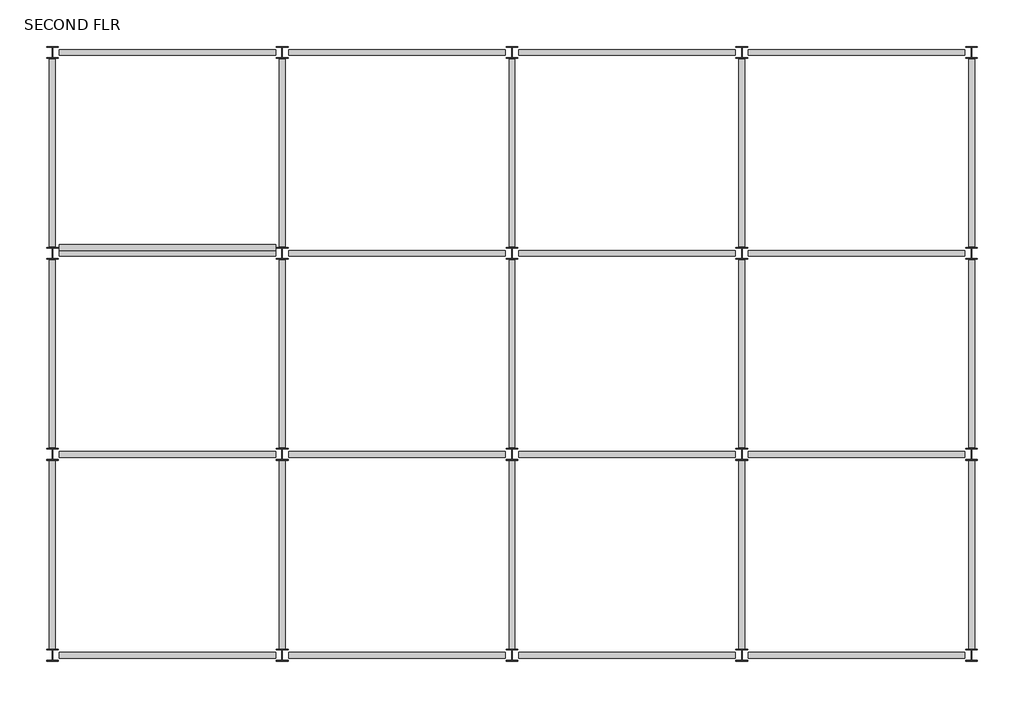
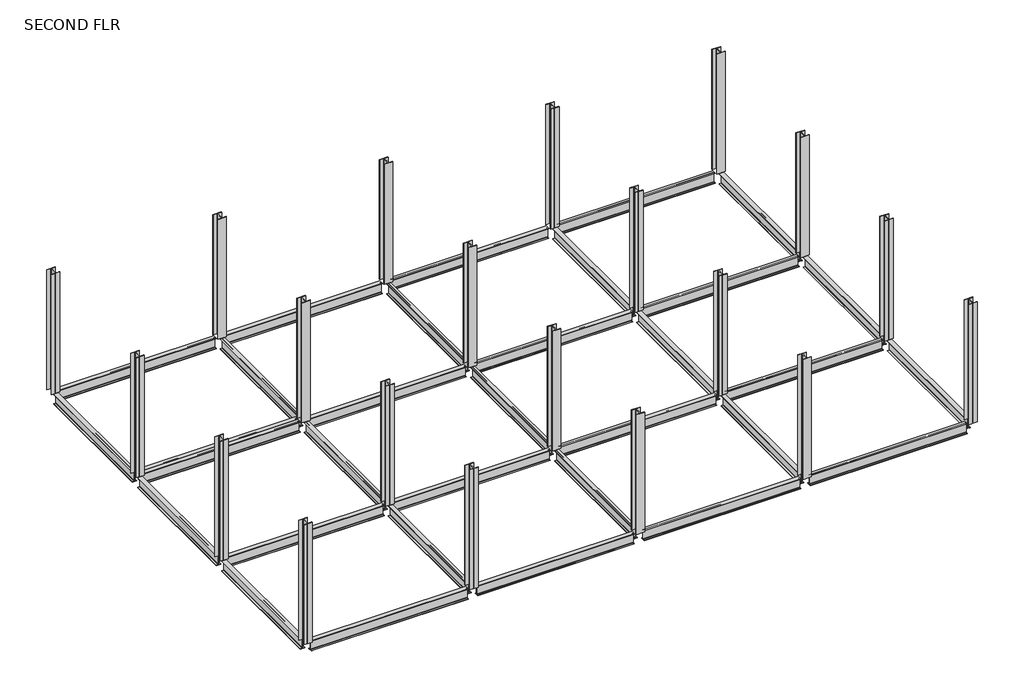
# One storey: 32 beams, 20 columns.
"""IFC4 building model written with IfcOpenShell, lengths in millimetres."""

from ifc_helpers import new_model, si_unit, origin, place, context, project, spatial, transform, mapped, element, save
from components import ub_universal_beams_ub254x102x28_022e5764, ub_universal_beams_ub254x102x28_3359efaf, ub_universal_beams_ub254x102x28_3001bc84, uc_universal_columns_column_uc203x203x52_01cb6b5e

model = new_model("IFC4")

# Units and contexts
model_context = context("Model", 3, world=origin())
ifc_project = project(units=[si_unit("LENGTHUNIT", "METRE", prefix="MILLI")], contexts=[model_context])

# Site, building, storey
site = spatial("IfcSite", under=ifc_project)
building = spatial("IfcBuilding", under=site)
storey = spatial("IfcBuildingStorey", under=building, Name="SECOND FLR", Elevation=6096.0)

# Beams
placement = place(None, origin())
ub_universal_beams_ub254x102x28_shape = ub_universal_beams_ub254x102x28_022e5764(model_context)
element("IfcBeam", 1, ObjectType="UB-Universal Beams : UB254x102x28", at=placement, inside=storey, context=model_context, shape_type="MappedRepresentation", body=[
    mapped(ub_universal_beams_ub254x102x28_shape, transform((-6871.2144105, 6458.2567898, 5965.8), x_axis=(1.0, 0.0, 0.0), y_axis=(0.0, 1.0, 0.0), z_axis=(0.0, 0.0, 1.0))),
])
ub_universal_beams_ub254x102x28_2_shape = ub_universal_beams_ub254x102x28_3359efaf(model_context)
element("IfcBeam", 2, ObjectType="UB-Universal Beams : UB254x102x28", at=placement, inside=storey, context=model_context, shape_type="MappedRepresentation", body=[
    mapped(ub_universal_beams_ub254x102x28_2_shape, transform((-8930.6620752, 1105.8028699, 5965.8), x_axis=(0.0, 1.0, 0.0), y_axis=(-1.0, 0.0, 0.0), z_axis=(0.0, 0.0, 1.0))),
])
element("IfcBeam", 3, ObjectType="UB-Universal Beams : UB254x102x28", at=placement, inside=storey, context=model_context, shape_type="MappedRepresentation", body=[
    mapped(ub_universal_beams_ub254x102x28_2_shape, transform((-8930.6620752, 4605.8028699, 5965.8), x_axis=(0.0, 1.0, 0.0), y_axis=(-1.0, 0.0, 0.0), z_axis=(0.0, 0.0, 1.0))),
])
element("IfcBeam", 4, ObjectType="UB-Universal Beams : UB254x102x28", at=placement, inside=storey, context=model_context, shape_type="MappedRepresentation", body=[
    mapped(ub_universal_beams_ub254x102x28_2_shape, transform((-8930.6620752, 8105.8028699, 5965.8), x_axis=(0.0, 1.0, 0.0), y_axis=(-1.0, 0.0, 0.0), z_axis=(0.0, 0.0, 1.0))),
])
element("IfcBeam", 5, ObjectType="UB-Universal Beams : UB254x102x28", at=placement, inside=storey, context=model_context, shape_type="MappedRepresentation", body=[
    mapped(ub_universal_beams_ub254x102x28_2_shape, transform((-4930.6620752, 1105.8028699, 5965.8), x_axis=(0.0, 1.0, 0.0), y_axis=(-1.0, 0.0, 0.0), z_axis=(0.0, 0.0, 1.0))),
])
element("IfcBeam", 6, ObjectType="UB-Universal Beams : UB254x102x28", at=placement, inside=storey, context=model_context, shape_type="MappedRepresentation", body=[
    mapped(ub_universal_beams_ub254x102x28_2_shape, transform((-4930.6620752, 4605.8028699, 5965.8), x_axis=(0.0, 1.0, 0.0), y_axis=(-1.0, 0.0, 0.0), z_axis=(0.0, 0.0, 1.0))),
])
element("IfcBeam", 7, ObjectType="UB-Universal Beams : UB254x102x28", at=placement, inside=storey, context=model_context, shape_type="MappedRepresentation", body=[
    mapped(ub_universal_beams_ub254x102x28_2_shape, transform((-4930.6620752, 8105.8028699, 5965.8), x_axis=(0.0, 1.0, 0.0), y_axis=(-1.0, 0.0, 0.0), z_axis=(0.0, 0.0, 1.0))),
])
element("IfcBeam", 8, ObjectType="UB-Universal Beams : UB254x102x28", at=placement, inside=storey, context=model_context, shape_type="MappedRepresentation", body=[
    mapped(ub_universal_beams_ub254x102x28_2_shape, transform((-930.6620752, 1105.8028699, 5965.8), x_axis=(0.0, 1.0, 0.0), y_axis=(-1.0, 0.0, 0.0), z_axis=(0.0, 0.0, 1.0))),
])
element("IfcBeam", 9, ObjectType="UB-Universal Beams : UB254x102x28", at=placement, inside=storey, context=model_context, shape_type="MappedRepresentation", body=[
    mapped(ub_universal_beams_ub254x102x28_2_shape, transform((-930.6620752, 4605.8028699, 5965.8), x_axis=(0.0, 1.0, 0.0), y_axis=(-1.0, 0.0, 0.0), z_axis=(0.0, 0.0, 1.0))),
])
element("IfcBeam", 10, ObjectType="UB-Universal Beams : UB254x102x28", at=placement, inside=storey, context=model_context, shape_type="MappedRepresentation", body=[
    mapped(ub_universal_beams_ub254x102x28_2_shape, transform((-930.6620752, 8105.8028699, 5965.8), x_axis=(0.0, 1.0, 0.0), y_axis=(-1.0, 0.0, 0.0), z_axis=(0.0, 0.0, 1.0))),
])
element("IfcBeam", 11, ObjectType="UB-Universal Beams : UB254x102x28", at=placement, inside=storey, context=model_context, shape_type="MappedRepresentation", body=[
    mapped(ub_universal_beams_ub254x102x28_2_shape, transform((3069.3379248, 1105.8028699, 5965.8), x_axis=(0.0, 1.0, 0.0), y_axis=(-1.0, 0.0, 0.0), z_axis=(0.0, 0.0, 1.0))),
])
element("IfcBeam", 12, ObjectType="UB-Universal Beams : UB254x102x28", at=placement, inside=storey, context=model_context, shape_type="MappedRepresentation", body=[
    mapped(ub_universal_beams_ub254x102x28_2_shape, transform((3069.3379248, 4605.8028699, 5965.8), x_axis=(0.0, 1.0, 0.0), y_axis=(-1.0, 0.0, 0.0), z_axis=(0.0, 0.0, 1.0))),
])
element("IfcBeam", 13, ObjectType="UB-Universal Beams : UB254x102x28", at=placement, inside=storey, context=model_context, shape_type="MappedRepresentation", body=[
    mapped(ub_universal_beams_ub254x102x28_2_shape, transform((3069.3379248, 8105.8028699, 5965.8), x_axis=(0.0, 1.0, 0.0), y_axis=(-1.0, 0.0, 0.0), z_axis=(0.0, 0.0, 1.0))),
])
element("IfcBeam", 14, ObjectType="UB-Universal Beams : UB254x102x28", at=placement, inside=storey, context=model_context, shape_type="MappedRepresentation", body=[
    mapped(ub_universal_beams_ub254x102x28_2_shape, transform((7069.3379248, 1105.8028699, 5965.8), x_axis=(0.0, 1.0, 0.0), y_axis=(-1.0, 0.0, 0.0), z_axis=(0.0, 0.0, 1.0))),
])
element("IfcBeam", 15, ObjectType="UB-Universal Beams : UB254x102x28", at=placement, inside=storey, context=model_context, shape_type="MappedRepresentation", body=[
    mapped(ub_universal_beams_ub254x102x28_2_shape, transform((7069.3379248, 4605.8028699, 5965.8), x_axis=(0.0, 1.0, 0.0), y_axis=(-1.0, 0.0, 0.0), z_axis=(0.0, 0.0, 1.0))),
])
element("IfcBeam", 16, ObjectType="UB-Universal Beams : UB254x102x28", at=placement, inside=storey, context=model_context, shape_type="MappedRepresentation", body=[
    mapped(ub_universal_beams_ub254x102x28_2_shape, transform((7069.3379248, 8105.8028699, 5965.8), x_axis=(0.0, 1.0, 0.0), y_axis=(-1.0, 0.0, 0.0), z_axis=(0.0, 0.0, 1.0))),
])
ub_universal_beams_ub254x102x28_3_shape = ub_universal_beams_ub254x102x28_3001bc84(model_context)
element("IfcBeam", 17, ObjectType="UB-Universal Beams : UB254x102x28", at=placement, inside=storey, context=model_context, shape_type="MappedRepresentation", body=[
    mapped(ub_universal_beams_ub254x102x28_3_shape, transform((-6930.6620752, 9855.8028699, 5965.8), x_axis=(1.0, 0.0, 0.0), y_axis=(0.0, 1.0, 0.0), z_axis=(0.0, 0.0, 1.0))),
])
element("IfcBeam", 18, ObjectType="UB-Universal Beams : UB254x102x28", at=placement, inside=storey, context=model_context, shape_type="MappedRepresentation", body=[
    mapped(ub_universal_beams_ub254x102x28_3_shape, transform((-2930.6620752, 9855.8028699, 5965.8), x_axis=(1.0, 0.0, 0.0), y_axis=(0.0, 1.0, 0.0), z_axis=(0.0, 0.0, 1.0))),
])
element("IfcBeam", 19, ObjectType="UB-Universal Beams : UB254x102x28", at=placement, inside=storey, context=model_context, shape_type="MappedRepresentation", body=[
    mapped(ub_universal_beams_ub254x102x28_3_shape, transform((1069.3379248, 9855.8028699, 5965.8), x_axis=(1.0, 0.0, 0.0), y_axis=(0.0, 1.0, 0.0), z_axis=(0.0, 0.0, 1.0))),
])
element("IfcBeam", 20, ObjectType="UB-Universal Beams : UB254x102x28", at=placement, inside=storey, context=model_context, shape_type="MappedRepresentation", body=[
    mapped(ub_universal_beams_ub254x102x28_3_shape, transform((5069.3379248, 9855.8028699, 5965.8), x_axis=(1.0, 0.0, 0.0), y_axis=(0.0, 1.0, 0.0), z_axis=(0.0, 0.0, 1.0))),
])
element("IfcBeam", 21, ObjectType="UB-Universal Beams : UB254x102x28", at=placement, inside=storey, context=model_context, shape_type="MappedRepresentation", body=[
    mapped(ub_universal_beams_ub254x102x28_3_shape, transform((-6930.6620752, 6355.8028699, 5965.8), x_axis=(1.0, 0.0, 0.0), y_axis=(0.0, 1.0, 0.0), z_axis=(0.0, 0.0, 1.0))),
])
element("IfcBeam", 22, ObjectType="UB-Universal Beams : UB254x102x28", at=placement, inside=storey, context=model_context, shape_type="MappedRepresentation", body=[
    mapped(ub_universal_beams_ub254x102x28_3_shape, transform((-2930.6620752, 6355.8028699, 5965.8), x_axis=(1.0, 0.0, 0.0), y_axis=(0.0, 1.0, 0.0), z_axis=(0.0, 0.0, 1.0))),
])
element("IfcBeam", 23, ObjectType="UB-Universal Beams : UB254x102x28", at=placement, inside=storey, context=model_context, shape_type="MappedRepresentation", body=[
    mapped(ub_universal_beams_ub254x102x28_3_shape, transform((1069.3379248, 6355.8028699, 5965.8), x_axis=(1.0, 0.0, 0.0), y_axis=(0.0, 1.0, 0.0), z_axis=(0.0, 0.0, 1.0))),
])
element("IfcBeam", 24, ObjectType="UB-Universal Beams : UB254x102x28", at=placement, inside=storey, context=model_context, shape_type="MappedRepresentation", body=[
    mapped(ub_universal_beams_ub254x102x28_3_shape, transform((5069.3379248, 6355.8028699, 5965.8), x_axis=(1.0, 0.0, 0.0), y_axis=(0.0, 1.0, 0.0), z_axis=(0.0, 0.0, 1.0))),
])
element("IfcBeam", 25, ObjectType="UB-Universal Beams : UB254x102x28", at=placement, inside=storey, context=model_context, shape_type="MappedRepresentation", body=[
    mapped(ub_universal_beams_ub254x102x28_3_shape, transform((-6930.6620752, 2855.8028699, 5965.8), x_axis=(1.0, 0.0, 0.0), y_axis=(0.0, 1.0, 0.0), z_axis=(0.0, 0.0, 1.0))),
])
element("IfcBeam", 26, ObjectType="UB-Universal Beams : UB254x102x28", at=placement, inside=storey, context=model_context, shape_type="MappedRepresentation", body=[
    mapped(ub_universal_beams_ub254x102x28_3_shape, transform((-2930.6620752, 2855.8028699, 5965.8), x_axis=(1.0, 0.0, 0.0), y_axis=(0.0, 1.0, 0.0), z_axis=(0.0, 0.0, 1.0))),
])
element("IfcBeam", 27, ObjectType="UB-Universal Beams : UB254x102x28", at=placement, inside=storey, context=model_context, shape_type="MappedRepresentation", body=[
    mapped(ub_universal_beams_ub254x102x28_3_shape, transform((1069.3379248, 2855.8028699, 5965.8), x_axis=(1.0, 0.0, 0.0), y_axis=(0.0, 1.0, 0.0), z_axis=(0.0, 0.0, 1.0))),
])
element("IfcBeam", 28, ObjectType="UB-Universal Beams : UB254x102x28", at=placement, inside=storey, context=model_context, shape_type="MappedRepresentation", body=[
    mapped(ub_universal_beams_ub254x102x28_3_shape, transform((5069.3379248, 2855.8028699, 5965.8), x_axis=(1.0, 0.0, 0.0), y_axis=(0.0, 1.0, 0.0), z_axis=(0.0, 0.0, 1.0))),
])
element("IfcBeam", 29, ObjectType="UB-Universal Beams : UB254x102x28", at=placement, inside=storey, context=model_context, shape_type="MappedRepresentation", body=[
    mapped(ub_universal_beams_ub254x102x28_3_shape, transform((-6930.6620752, -644.1971301, 5965.8), x_axis=(1.0, 0.0, 0.0), y_axis=(0.0, 1.0, 0.0), z_axis=(0.0, 0.0, 1.0))),
])
element("IfcBeam", 30, ObjectType="UB-Universal Beams : UB254x102x28", at=placement, inside=storey, context=model_context, shape_type="MappedRepresentation", body=[
    mapped(ub_universal_beams_ub254x102x28_3_shape, transform((-2930.6620752, -644.1971301, 5965.8), x_axis=(1.0, 0.0, 0.0), y_axis=(0.0, 1.0, 0.0), z_axis=(0.0, 0.0, 1.0))),
])
element("IfcBeam", 31, ObjectType="UB-Universal Beams : UB254x102x28", at=placement, inside=storey, context=model_context, shape_type="MappedRepresentation", body=[
    mapped(ub_universal_beams_ub254x102x28_3_shape, transform((1069.3379248, -644.1971301, 5965.8), x_axis=(1.0, 0.0, 0.0), y_axis=(0.0, 1.0, 0.0), z_axis=(0.0, 0.0, 1.0))),
])
element("IfcBeam", 32, ObjectType="UB-Universal Beams : UB254x102x28", at=placement, inside=storey, context=model_context, shape_type="MappedRepresentation", body=[
    mapped(ub_universal_beams_ub254x102x28_3_shape, transform((5069.3379248, -644.1971301, 5965.8), x_axis=(1.0, 0.0, 0.0), y_axis=(0.0, 1.0, 0.0), z_axis=(0.0, 0.0, 1.0))),
])

# Columns
uc_universal_columns_column_uc203x203x52_shape = uc_universal_columns_column_uc203x203x52_01cb6b5e(model_context)
element("IfcColumn", 33, ObjectType="UC-Universal Columns-Column : UC203x203x52", at=placement, inside=storey, context=model_context, shape_type="MappedRepresentation", body=[
    mapped(uc_universal_columns_column_uc203x203x52_shape, transform((-8930.6620752, 9855.8028699, 0.0), x_axis=(1.0, 0.0, 0.0), y_axis=(0.0, 1.0, 0.0), z_axis=(0.0, 0.0, 1.0))),
])
element("IfcColumn", 34, ObjectType="UC-Universal Columns-Column : UC203x203x52", at=placement, inside=storey, context=model_context, shape_type="MappedRepresentation", body=[
    mapped(uc_universal_columns_column_uc203x203x52_shape, transform((-8930.6620752, 6355.8028699, 0.0), x_axis=(1.0, 0.0, 0.0), y_axis=(0.0, 1.0, 0.0), z_axis=(0.0, 0.0, 1.0))),
])
element("IfcColumn", 35, ObjectType="UC-Universal Columns-Column : UC203x203x52", at=placement, inside=storey, context=model_context, shape_type="MappedRepresentation", body=[
    mapped(uc_universal_columns_column_uc203x203x52_shape, transform((-8930.6620752, 2855.8028699, 0.0), x_axis=(1.0, 0.0, 0.0), y_axis=(0.0, 1.0, 0.0), z_axis=(0.0, 0.0, 1.0))),
])
element("IfcColumn", 36, ObjectType="UC-Universal Columns-Column : UC203x203x52", at=placement, inside=storey, context=model_context, shape_type="MappedRepresentation", body=[
    mapped(uc_universal_columns_column_uc203x203x52_shape, transform((-8930.6620752, -644.1971301, 0.0), x_axis=(1.0, 0.0, 0.0), y_axis=(0.0, 1.0, 0.0), z_axis=(0.0, 0.0, 1.0))),
])
element("IfcColumn", 37, ObjectType="UC-Universal Columns-Column : UC203x203x52", at=placement, inside=storey, context=model_context, shape_type="MappedRepresentation", body=[
    mapped(uc_universal_columns_column_uc203x203x52_shape, transform((-4930.6620752, 9855.8028699, 0.0), x_axis=(1.0, 0.0, 0.0), y_axis=(0.0, 1.0, 0.0), z_axis=(0.0, 0.0, 1.0))),
])
element("IfcColumn", 38, ObjectType="UC-Universal Columns-Column : UC203x203x52", at=placement, inside=storey, context=model_context, shape_type="MappedRepresentation", body=[
    mapped(uc_universal_columns_column_uc203x203x52_shape, transform((-4930.6620752, 6355.8028699, 0.0), x_axis=(1.0, 0.0, 0.0), y_axis=(0.0, 1.0, 0.0), z_axis=(0.0, 0.0, 1.0))),
])
element("IfcColumn", 39, ObjectType="UC-Universal Columns-Column : UC203x203x52", at=placement, inside=storey, context=model_context, shape_type="MappedRepresentation", body=[
    mapped(uc_universal_columns_column_uc203x203x52_shape, transform((-4930.6620752, 2855.8028699, 0.0), x_axis=(1.0, 0.0, 0.0), y_axis=(0.0, 1.0, 0.0), z_axis=(0.0, 0.0, 1.0))),
])
element("IfcColumn", 40, ObjectType="UC-Universal Columns-Column : UC203x203x52", at=placement, inside=storey, context=model_context, shape_type="MappedRepresentation", body=[
    mapped(uc_universal_columns_column_uc203x203x52_shape, transform((-4930.6620752, -644.1971301, 0.0), x_axis=(1.0, 0.0, 0.0), y_axis=(0.0, 1.0, 0.0), z_axis=(0.0, 0.0, 1.0))),
])
element("IfcColumn", 41, ObjectType="UC-Universal Columns-Column : UC203x203x52", at=placement, inside=storey, context=model_context, shape_type="MappedRepresentation", body=[
    mapped(uc_universal_columns_column_uc203x203x52_shape, transform((-930.6620752, 9855.8028699, 0.0), x_axis=(1.0, 0.0, 0.0), y_axis=(0.0, 1.0, 0.0), z_axis=(0.0, 0.0, 1.0))),
])
element("IfcColumn", 42, ObjectType="UC-Universal Columns-Column : UC203x203x52", at=placement, inside=storey, context=model_context, shape_type="MappedRepresentation", body=[
    mapped(uc_universal_columns_column_uc203x203x52_shape, transform((-930.6620752, 6355.8028699, 0.0), x_axis=(1.0, 0.0, 0.0), y_axis=(0.0, 1.0, 0.0), z_axis=(0.0, 0.0, 1.0))),
])
element("IfcColumn", 43, ObjectType="UC-Universal Columns-Column : UC203x203x52", at=placement, inside=storey, context=model_context, shape_type="MappedRepresentation", body=[
    mapped(uc_universal_columns_column_uc203x203x52_shape, transform((-930.6620752, 2855.8028699, 0.0), x_axis=(1.0, 0.0, 0.0), y_axis=(0.0, 1.0, 0.0), z_axis=(0.0, 0.0, 1.0))),
])
element("IfcColumn", 44, ObjectType="UC-Universal Columns-Column : UC203x203x52", at=placement, inside=storey, context=model_context, shape_type="MappedRepresentation", body=[
    mapped(uc_universal_columns_column_uc203x203x52_shape, transform((-930.6620752, -644.1971301, 0.0), x_axis=(1.0, 0.0, 0.0), y_axis=(0.0, 1.0, 0.0), z_axis=(0.0, 0.0, 1.0))),
])
element("IfcColumn", 45, ObjectType="UC-Universal Columns-Column : UC203x203x52", at=placement, inside=storey, context=model_context, shape_type="MappedRepresentation", body=[
    mapped(uc_universal_columns_column_uc203x203x52_shape, transform((3069.3379248, 9855.8028699, 0.0), x_axis=(1.0, 0.0, 0.0), y_axis=(0.0, 1.0, 0.0), z_axis=(0.0, 0.0, 1.0))),
])
element("IfcColumn", 46, ObjectType="UC-Universal Columns-Column : UC203x203x52", at=placement, inside=storey, context=model_context, shape_type="MappedRepresentation", body=[
    mapped(uc_universal_columns_column_uc203x203x52_shape, transform((3069.3379248, 6355.8028699, 0.0), x_axis=(1.0, 0.0, 0.0), y_axis=(0.0, 1.0, 0.0), z_axis=(0.0, 0.0, 1.0))),
])
element("IfcColumn", 47, ObjectType="UC-Universal Columns-Column : UC203x203x52", at=placement, inside=storey, context=model_context, shape_type="MappedRepresentation", body=[
    mapped(uc_universal_columns_column_uc203x203x52_shape, transform((3069.3379248, 2855.8028699, 0.0), x_axis=(1.0, 0.0, 0.0), y_axis=(0.0, 1.0, 0.0), z_axis=(0.0, 0.0, 1.0))),
])
element("IfcColumn", 48, ObjectType="UC-Universal Columns-Column : UC203x203x52", at=placement, inside=storey, context=model_context, shape_type="MappedRepresentation", body=[
    mapped(uc_universal_columns_column_uc203x203x52_shape, transform((3069.3379248, -644.1971301, 0.0), x_axis=(1.0, 0.0, 0.0), y_axis=(0.0, 1.0, 0.0), z_axis=(0.0, 0.0, 1.0))),
])
element("IfcColumn", 49, ObjectType="UC-Universal Columns-Column : UC203x203x52", at=placement, inside=storey, context=model_context, shape_type="MappedRepresentation", body=[
    mapped(uc_universal_columns_column_uc203x203x52_shape, transform((7069.3379248, 9855.8028699, 0.0), x_axis=(1.0, 0.0, 0.0), y_axis=(0.0, 1.0, 0.0), z_axis=(0.0, 0.0, 1.0))),
])
element("IfcColumn", 50, ObjectType="UC-Universal Columns-Column : UC203x203x52", at=placement, inside=storey, context=model_context, shape_type="MappedRepresentation", body=[
    mapped(uc_universal_columns_column_uc203x203x52_shape, transform((7069.3379248, 6355.8028699, 0.0), x_axis=(1.0, 0.0, 0.0), y_axis=(0.0, 1.0, 0.0), z_axis=(0.0, 0.0, 1.0))),
])
element("IfcColumn", 51, ObjectType="UC-Universal Columns-Column : UC203x203x52", at=placement, inside=storey, context=model_context, shape_type="MappedRepresentation", body=[
    mapped(uc_universal_columns_column_uc203x203x52_shape, transform((7069.3379248, 2855.8028699, 0.0), x_axis=(1.0, 0.0, 0.0), y_axis=(0.0, 1.0, 0.0), z_axis=(0.0, 0.0, 1.0))),
])
element("IfcColumn", 52, ObjectType="UC-Universal Columns-Column : UC203x203x52", at=placement, inside=storey, context=model_context, shape_type="MappedRepresentation", body=[
    mapped(uc_universal_columns_column_uc203x203x52_shape, transform((7069.3379248, -644.1971301, 0.0), x_axis=(1.0, 0.0, 0.0), y_axis=(0.0, 1.0, 0.0), z_axis=(0.0, 0.0, 1.0))),
])

save(model, "model.ifc")

# Revit data of these elements
# Type "UB-Universal Beams : UB254x102x28"
#   Section Name Key = "UB254X102X28"
#   Width = 10.22 cm
#   Web Thickness = 0.63 cm
#   Web Fillet = 0.76 cm
#   Warping Constant = 28000.0 cm⁶
#   Torsional Moment of Inertia = 9.57 cm⁴
#   Section Area = 36.1 cm²
#   Plastic Modulus weak axis = 54.8 cm³
#   Plastic Modulus strong axis = 353.0 cm³
#   Nominal Weight = 28.2999 kgf/m
#   Moment of Inertia weak axis = 179.00 cm⁴
#   Moment of Inertia strong axis = 4005.00 cm⁴
#   Height = 26.04 cm
#   Flange Thickness = 1.0 cm
#   Elastic Modulus weak axis = 34.9 cm³
#   Elastic Modulus strong axis = 308.0 cm³
#   Centroid Vertical = 13.02 cm
#   Centroid Horizontal = 5.11 cm
#   Bolt Spacing = 5.4 cm
#   Length [instance default] = 4' - 11.05512"
#   Structural Material [instance default] = Metal - Steel 43-275
#   Type Comments = ""
#   Assembly Code = ""
# Type "UC-Universal Columns-Column : UC203x203x52"
#   Section Name Key = "UC203x203x52"
#   Width = 20.43 cm
#   Web Thickness = 0.79 cm
#   Web Fillet = 1.02 cm
#   Warping Constant = 167000.0 cm⁶
#   Torsional Moment of Inertia = 31.80 cm⁴
#   Section Area = 66.0 cm²
#   Plastic Modulus weak axis = 264.0 cm³
#   Plastic Modulus strong axis = 567.0 cm³
#   Nominal Weight = 51.9998 kgf/m
#   Moment of Inertia weak axis = 1778.00 cm⁴
#   Moment of Inertia strong axis = 5259.00 cm⁴
#   Height = 20.62 cm
#   Flange Thickness = 1.25 cm
#   Elastic Modulus weak axis = 174.0 cm³
#   Elastic Modulus strong axis = 510.0 cm³
#   Centroid Vertical = 10.31 cm
#   Centroid Horizontal = 10.215 cm
#   Bolt Spacing = 14.0 cm
#   Structural Material [instance default] = Metal - Steel 43-275
#   Type Comments = ""
#   Assembly Code = ""
# Elements 1, 2, 3, 4, 5, 6, 7, 8, 9, 10, 11, 12, 13, 14, 15, 16, 17, 18, 19, 20, 21, 22, 23, 24, 25, 26, 27, 28, 29, 30, 31, 32 (IfcBeam, "UB-Universal Beams : UB254x102x28")
#   Structural Material = Metal - Steel 43-275
#   Phase Created = New Construction
#   Materials on its faces: "Metal - Steel 43-275"
# Elements 33, 34, 35, 36, 37, 38, 39, 40, 41, 42, 43, 44, 45, 46, 47, 48, 49, 50, 51, 52 (IfcColumn, "UC-Universal Columns-Column : UC203x203x52")
#   Structural Material = Metal - Steel 43-275
#   Phase Created = New Construction
#   Materials on its faces: "Metal - Steel 43-275"
# Materials
#   "Metal - Steel 43-275": class "Metal", colour RGB 247 247 247, transparency 0, Cost = 0
